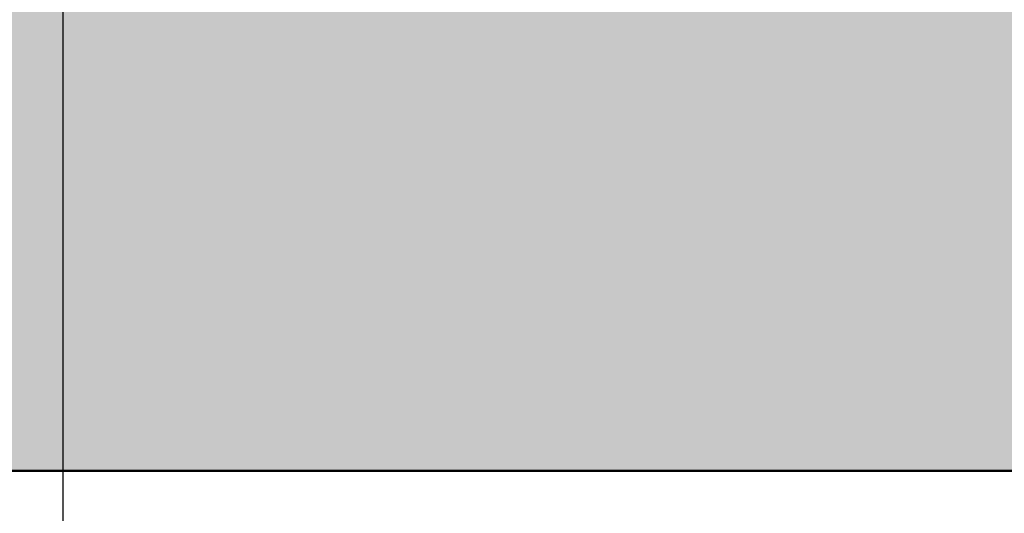
# Model space of a CAD drawing. Units: millimetres. Extents: x 0 to 2267, y 0 to 1823.
# Tile 24 of 256: x 1590 to 1675, y 1074 to 1117. Entities that reach past the tile are written whole.
import ezdxf

# ---------------------------------------------------------------- set-up
doc = ezdxf.new("R2010")
doc.units = ezdxf.units.MM
doc.header["$MEASUREMENT"] = 0
for name, color, linetype, lineweight in [('M-DIMS', 2, 'Continuous', 25), ('M-HATC', 252, 'Continuous', 18), ('M-OUTL', 7, 'Continuous', 50)]:
    doc.layers.add(name, color=color, linetype=linetype, lineweight=lineweight)
doc.styles.get("Standard").update_dxf_attribs({"font": 'arial.ttf'})
doc.dimstyles.get("Standard").update_dxf_attribs({"dimtxt": 7, "dimasz": 4, "dimexe": 0.18, "dimexo": 0.0625, "dimgap": 0.09, "dimtad": 0, "dimdec": 0, "dimzin": 0, "dimdsep": 46, "dimtxsty": 'Standard', "dimcen": 0.09, "dimadec": 0, "dimazin": 0, "dimtfac": 1, "dimtdec": 0, "dimtofl": 0, "dimtmove": 0, "dimatfit": 3, "dimfxl": 1, "dimtolj": 1, "dimtzin": 0, "dimarcsym": 0})

# ---------------------------------------------------------------- blocks, each defined once
blk = doc.blocks.new('*D1')
at = {"layer": 'Defpoints', "color": 0, "transparency": 16777216}
for p in [(1593.429, 1127.417), (1843.429, 1127.417), (1843.429, 955.628)]:
    blk.add_point(p, dxfattribs=at)
at = {"layer": 'M-DIMS', "color": 0, "lineweight": -2, "transparency": 16777216}
for p, q in [((1593.429, 1127.355), (1593.429, 955.448)), ((1843.429, 1127.355), (1843.429, 955.448)), ((1597.429, 955.628), (1710.558, 955.628)), ((1839.429, 955.628), (1726.3, 955.628))]:
    blk.add_line(p, q, dxfattribs=at)
at = {"layer": 'M-DIMS', "color": 0, "transparency": 16777216}
for points in [[(1597.429, 956.294), (1597.429, 954.961), (1593.429, 955.628)], [(1839.429, 956.294), (1839.429, 954.961), (1843.429, 955.628)]]:
    blk.add_solid(points, dxfattribs=at)
at = {"layer": 'M-DIMS', "color": 0, "transparency": 16777216, "insert": (1718.429, 955.628), "char_height": 7, "attachment_point": 5}
blk.add_mtext('\\A1;250', dxfattribs=at)
blk = doc.blocks.new('*D2')
at = {"layer": 'Defpoints', "color": 0, "transparency": 16777216}
for p in [(1505.929, 1077.417), (1930.929, 1077.417), (1930.929, 906.787)]:
    blk.add_point(p, dxfattribs=at)
at = {"layer": 'M-DIMS', "color": 0, "lineweight": -2, "transparency": 16777216}
for p, q in [((1505.929, 1077.355), (1505.929, 906.607)), ((1930.929, 1077.355), (1930.929, 906.607)), ((1509.929, 906.787), (1710.439, 906.787)), ((1926.929, 906.787), (1726.419, 906.787))]:
    blk.add_line(p, q, dxfattribs=at)
at = {"layer": 'M-DIMS', "color": 0, "transparency": 16777216}
for points in [[(1509.929, 907.453), (1509.929, 906.12), (1505.929, 906.787)], [(1926.929, 907.453), (1926.929, 906.12), (1930.929, 906.787)]]:
    blk.add_solid(points, dxfattribs=at)
at = {"layer": 'M-DIMS', "color": 0, "transparency": 16777216, "insert": (1718.429, 906.787), "char_height": 7, "attachment_point": 5}
blk.add_mtext('\\A1;425', dxfattribs=at)

msp = doc.modelspace()

# ---------------------------------------------------------------- hatches: boundary and pattern name
at = {"layer": 'M-HATC'}
h = msp.add_hatch(color=256, dxfattribs=at)
h.dxf.hatch_style = 1
h.paths.add_polyline_path([(2065.771, 1618.062, 0.236068), (2055.771, 1638.062), (1381.087, 1638.062, 0.236068), (1371.087, 1618.062), (1371.087, 1603.062), (2055.771, 1603.062), (2065.771, 1603.062)])
h.paths.add_polyline_path([(2062.772, 1550.296), (2062.772, 1560.296), (1374.086, 1560.296), (1374.086, 1550.296), (1374.086, 1540.296), (1384.086, 1540.296), (1389.086, 1540.296), (2062.772, 1540.296)])
h.paths.add_polyline_path([(1930.929, 1282.766), (1505.929, 1282.766), (1587.628, 1235.597, 0.131652), (1600.128, 1232.247), (1836.73, 1232.247, 0.131652), (1849.23, 1235.597)])
h.paths.add_polyline_path([(1930.929, 1117.417), (1905.929, 1117.417), (1505.929, 1117.417), (1505.929, 1077.417), (1930.929, 1077.417)])

# ---------------------------------------------------------------- linework, layer by layer
at = {"layer": 'M-OUTL'}
msp.add_line((1505.929, 1077.417), (1930.929, 1077.417), dxfattribs=at)

# ---------------------------------------------------------------- dimensions: what is measured, and where the dimension line sits
at = {"layer": 'M-DIMS'}
for base, p1, p2, picture, middle in [((1843.429, 955.628), (1593.429, 1127.417), (1843.429, 1127.417), '*D1', (1718.429, 955.628)), ((1930.929, 906.787), (1505.929, 1077.417), (1930.929, 1077.417), '*D2', (1718.429, 906.787))]:
    dim = msp.add_linear_dim(base=base, p1=p1, p2=p2, dimstyle='Standard', override={"dimclrd": 0, "dimclre": 0, "dimclrt": 0}, dxfattribs=at)
    dim.commit()
    dim.dimension.update_dxf_attribs({"geometry": picture, "text_midpoint": middle})

doc.saveas('drawing.dxf')
